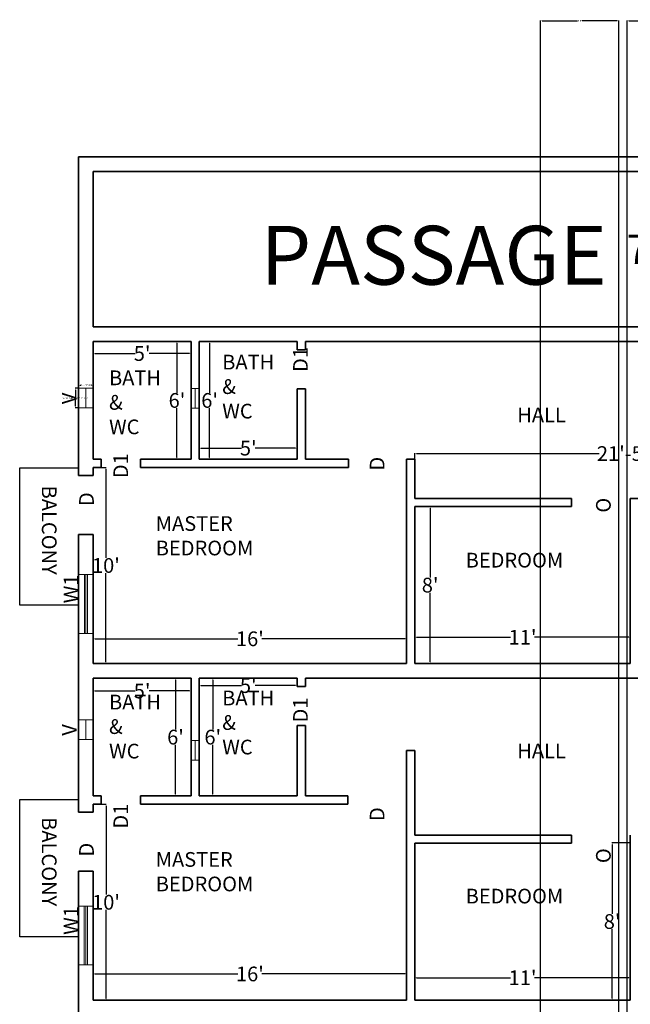
# Model space of a CAD drawing. Units: inches. Extents: x -2189 to 546, y 945 to 2684.
# Tile 4 of 10: x -866 to -492, y 2082 to 2684. Entities that reach past the tile are written whole.
import ezdxf

# ---------------------------------------------------------------- set-up
doc = ezdxf.new("R2010")
doc.units = ezdxf.units.IN
doc.header["$MEASUREMENT"] = 0
for name, color, linetype, lineweight in [('A-ANNO-DIMS', 2, 'Continuous', 13), ('A-ANNO-TEXT', 7, 'Continuous', 18), ('A-AREA-IDEN', 3, 'Continuous', 18), ('A-FLOR-BALC', 8, 'Continuous', 25), ('A-GLAZ', 4, 'Continuous', 18), ('A-WALL', 7, 'Continuous', 35)]:
    doc.layers.add(name, color=color, linetype=linetype, lineweight=lineweight)
doc.styles.get("Standard").update_dxf_attribs({"font": 'arial.ttf'})
doc.dimstyles.get("Standard").update_dxf_attribs({"dimtxt": 1, "dimasz": 1, "dimexe": 0.18, "dimexo": 0.0625, "dimgap": 0.09, "dimtad": 0, "dimtih": 1, "dimtoh": 1, "dimdec": 0, "dimzin": 0, "dimdsep": 46, "dimlunit": 3, "dimtxsty": 'Standard', "dimcen": 0.09, "dimadec": 0, "dimazin": 0, "dimtfac": 1, "dimtdec": 0, "dimtofl": 0, "dimtmove": 0, "dimatfit": 3, "dimfxl": 1, "dimtolj": 1, "dimtzin": 0, "dimarcsym": 0})

# ---------------------------------------------------------------- blocks, each defined once
blk = doc.blocks.new('*D57')
at = {"layer": 'A-ANNO-DIMS', "color": 0, "lineweight": -2, "transparency": 16777216}
for p, q in [((-820.78, 2084.24), (-820.78, 2100.43)), ((-819.78, 2100.25), (-732.08, 2100.25)), ((-629.78, 2100.25), (-717.48, 2100.25)), ((-628.78, 2084.24), (-628.78, 2100.43))]:
    blk.add_line(p, q, dxfattribs=at)
at = {"layer": 'A-ANNO-DIMS', "color": 0, "transparency": 16777216}
for points in [[(-819.78, 2100.42), (-819.78, 2100.08), (-820.78, 2100.25)], [(-629.78, 2100.42), (-629.78, 2100.08), (-628.78, 2100.25)]]:
    blk.add_solid(points, dxfattribs=at)
at = {"layer": 'Defpoints', "color": 0, "transparency": 16777216}
for p in [(-820.78, 2100.25), (-820.78, 2084.17), (-628.78, 2084.17)]:
    blk.add_point(p, dxfattribs=at)
at = {"layer": 'A-ANNO-DIMS', "color": 0, "transparency": 16777216, "insert": (-724.78, 2100.25), "char_height": 1, "attachment_point": 5}
blk.add_mtext("\\A1;{\\H9x;16'}", dxfattribs=at)
blk = doc.blocks.new('*D58')
at = {"layer": 'A-ANNO-DIMS', "color": 0, "lineweight": -2, "transparency": 16777216}
for p, q in [((-623.78, 2084.24), (-623.78, 2098.13)), ((-622.78, 2097.95), (-565.08, 2097.95)), ((-492.78, 2097.95), (-550.48, 2097.95)), ((-491.78, 2084.24), (-491.78, 2098.13))]:
    blk.add_line(p, q, dxfattribs=at)
at = {"layer": 'A-ANNO-DIMS', "color": 0, "transparency": 16777216}
for points in [[(-622.78, 2098.12), (-622.78, 2097.78), (-623.78, 2097.95)], [(-492.78, 2098.12), (-492.78, 2097.78), (-491.78, 2097.95)]]:
    blk.add_solid(points, dxfattribs=at)
at = {"layer": 'Defpoints', "color": 0, "transparency": 16777216}
for p in [(-623.78, 2097.95), (-623.78, 2084.17), (-491.78, 2084.17)]:
    blk.add_point(p, dxfattribs=at)
at = {"layer": 'A-ANNO-DIMS', "color": 0, "transparency": 16777216, "insert": (-557.78, 2097.95), "char_height": 1, "attachment_point": 5}
blk.add_mtext("\\A1;{\\H9x;11'}", dxfattribs=at)
blk = doc.blocks.new('*D61')
at = {"layer": 'A-ANNO-DIMS', "color": 0, "lineweight": -2, "transparency": 16777216}
for p, q in [((-820.78, 2281.11), (-820.78, 2273.2)), ((-760.78, 2281.11), (-760.78, 2273.2)), ((-819.78, 2273.38), (-795.01, 2273.38)), ((-761.78, 2273.38), (-786.55, 2273.38))]:
    blk.add_line(p, q, dxfattribs=at)
at = {"layer": 'A-ANNO-DIMS', "color": 0, "transparency": 16777216}
for points in [[(-819.78, 2273.55), (-819.78, 2273.22), (-820.78, 2273.38)], [(-761.78, 2273.55), (-761.78, 2273.22), (-760.78, 2273.38)]]:
    blk.add_solid(points, dxfattribs=at)
at = {"layer": 'Defpoints', "color": 0, "transparency": 16777216}
for p in [(-820.78, 2281.17), (-760.78, 2281.17), (-820.78, 2273.38)]:
    blk.add_point(p, dxfattribs=at)
at = {"layer": 'A-ANNO-DIMS', "color": 0, "transparency": 16777216, "insert": (-790.78, 2273.38), "char_height": 1, "attachment_point": 5}
blk.add_mtext("\\A1;{\\H9x;5'}", dxfattribs=at)
blk = doc.blocks.new('*D62')
at = {"layer": 'A-ANNO-DIMS', "color": 0, "lineweight": -2, "transparency": 16777216}
for p, q in [((-760.84, 2281.17), (-770.51, 2281.17)), ((-770.33, 2280.17), (-770.33, 2249.86)), ((-770.33, 2210.17), (-770.33, 2240.49)), ((-760.84, 2209.17), (-770.51, 2209.17))]:
    blk.add_line(p, q, dxfattribs=at)
at = {"layer": 'A-ANNO-DIMS', "color": 0, "transparency": 16777216}
for points in [[(-770.5, 2280.17), (-770.17, 2280.17), (-770.33, 2281.17)], [(-770.5, 2210.17), (-770.17, 2210.17), (-770.33, 2209.17)]]:
    blk.add_solid(points, dxfattribs=at)
at = {"layer": 'Defpoints', "color": 0, "transparency": 16777216}
for p in [(-770.33, 2281.17), (-760.78, 2281.17), (-760.78, 2209.17)]:
    blk.add_point(p, dxfattribs=at)
at = {"layer": 'A-ANNO-DIMS', "color": 0, "transparency": 16777216, "insert": (-770.33, 2245.17), "char_height": 1, "attachment_point": 5}
blk.add_mtext("\\A1;{\\H9x;6'}", dxfattribs=at)
blk = doc.blocks.new('*D63')
at = {"layer": 'A-ANNO-DIMS', "color": 0, "lineweight": -2, "transparency": 16777216}
for p, q in [((-755.72, 2281.17), (-747.34, 2281.17)), ((-747.52, 2280.17), (-747.52, 2249.86)), ((-747.52, 2210.17), (-747.52, 2240.49)), ((-755.72, 2209.17), (-747.34, 2209.17))]:
    blk.add_line(p, q, dxfattribs=at)
at = {"layer": 'A-ANNO-DIMS', "color": 0, "transparency": 16777216}
for points in [[(-747.69, 2280.17), (-747.35, 2280.17), (-747.52, 2281.17)], [(-747.69, 2210.17), (-747.35, 2210.17), (-747.52, 2209.17)]]:
    blk.add_solid(points, dxfattribs=at)
at = {"layer": 'Defpoints', "color": 0, "transparency": 16777216}
for p in [(-755.78, 2281.17), (-747.52, 2281.17), (-755.78, 2209.17)]:
    blk.add_point(p, dxfattribs=at)
at = {"layer": 'A-ANNO-DIMS', "color": 0, "transparency": 16777216, "insert": (-747.52, 2245.17), "char_height": 1, "attachment_point": 5}
blk.add_mtext("\\A1;{\\H9x;6'}", dxfattribs=at)
blk = doc.blocks.new('*D64')
at = {"layer": 'A-ANNO-DIMS', "color": 0, "lineweight": -2, "transparency": 16777216}
for p, q in [((-755.78, 2281.11), (-755.78, 2276.52)), ((-695.78, 2281.11), (-695.78, 2276.52)), ((-754.78, 2276.7), (-730.01, 2276.7)), ((-696.78, 2276.7), (-721.55, 2276.7))]:
    blk.add_line(p, q, dxfattribs=at)
at = {"layer": 'A-ANNO-DIMS', "color": 0, "transparency": 16777216}
for points in [[(-754.78, 2276.86), (-754.78, 2276.53), (-755.78, 2276.7)], [(-696.78, 2276.86), (-696.78, 2276.53), (-695.78, 2276.7)]]:
    blk.add_solid(points, dxfattribs=at)
at = {"layer": 'Defpoints', "color": 0, "transparency": 16777216}
for p in [(-755.78, 2281.17), (-695.78, 2281.17), (-755.78, 2276.7)]:
    blk.add_point(p, dxfattribs=at)
at = {"layer": 'A-ANNO-DIMS', "color": 0, "transparency": 16777216, "insert": (-725.78, 2276.7), "char_height": 1, "attachment_point": 5}
blk.add_mtext("\\A1;{\\H9x;5'}", dxfattribs=at)
blk = doc.blocks.new('*D65')
at = {"layer": 'A-ANNO-DIMS', "color": 0, "lineweight": -2, "transparency": 16777216}
for p, q in [((-820.75, 2204.04), (-812.72, 2204.04)), ((-812.9, 2203.04), (-812.9, 2148.8)), ((-812.9, 2085.19), (-812.9, 2139.43)), ((-820.75, 2084.19), (-812.72, 2084.19))]:
    blk.add_line(p, q, dxfattribs=at)
at = {"layer": 'A-ANNO-DIMS', "color": 0, "transparency": 16777216}
for points in [[(-813.07, 2203.04), (-812.73, 2203.04), (-812.9, 2204.04)], [(-813.07, 2085.19), (-812.73, 2085.19), (-812.9, 2084.19)]]:
    blk.add_solid(points, dxfattribs=at)
at = {"layer": 'Defpoints', "color": 0, "transparency": 16777216}
for p in [(-820.82, 2204.04), (-820.82, 2084.19), (-812.9, 2084.19)]:
    blk.add_point(p, dxfattribs=at)
at = {"layer": 'A-ANNO-DIMS', "color": 0, "transparency": 16777216, "insert": (-812.9, 2144.11), "char_height": 1, "attachment_point": 5}
blk.add_mtext("\\A1;{\\H9x;10'}", dxfattribs=at)
blk = doc.blocks.new('*D66')
at = {"layer": 'A-ANNO-DIMS', "color": 0, "lineweight": -2, "transparency": 16777216}
for p, q in [((-491.84, 2180.47), (-503.11, 2180.47)), ((-502.93, 2179.47), (-502.93, 2137.01)), ((-502.93, 2085.17), (-502.93, 2127.64)), ((-491.84, 2084.17), (-503.11, 2084.17))]:
    blk.add_line(p, q, dxfattribs=at)
at = {"layer": 'A-ANNO-DIMS', "color": 0, "transparency": 16777216}
for points in [[(-503.1, 2179.47), (-502.76, 2179.47), (-502.93, 2180.47)], [(-503.1, 2085.17), (-502.76, 2085.17), (-502.93, 2084.17)]]:
    blk.add_solid(points, dxfattribs=at)
at = {"layer": 'Defpoints', "color": 0, "transparency": 16777216}
for p in [(-491.78, 2180.47), (-502.93, 2084.17), (-491.78, 2084.17)]:
    blk.add_point(p, dxfattribs=at)
at = {"layer": 'A-ANNO-DIMS', "color": 0, "transparency": 16777216, "insert": (-502.93, 2132.32), "char_height": 1, "attachment_point": 5}
blk.add_mtext("\\A1;{\\H9x;8'}", dxfattribs=at)
blk = doc.blocks.new('*D67')
at = {"layer": 'A-ANNO-DIMS', "color": 0, "lineweight": -2, "transparency": 16777216}
for p, q in [((-820.78, 2290.24), (-820.78, 2305.51)), ((-819.78, 2305.33), (-732.08, 2305.33)), ((-629.78, 2305.33), (-717.48, 2305.33)), ((-628.78, 2290.24), (-628.78, 2305.51))]:
    blk.add_line(p, q, dxfattribs=at)
at = {"layer": 'A-ANNO-DIMS', "color": 0, "transparency": 16777216}
for points in [[(-819.78, 2305.5), (-819.78, 2305.17), (-820.78, 2305.33)], [(-629.78, 2305.5), (-629.78, 2305.17), (-628.78, 2305.33)]]:
    blk.add_solid(points, dxfattribs=at)
at = {"layer": 'Defpoints', "color": 0, "transparency": 16777216}
for p in [(-820.78, 2305.33), (-820.78, 2290.17), (-628.78, 2290.17)]:
    blk.add_point(p, dxfattribs=at)
at = {"layer": 'A-ANNO-DIMS', "color": 0, "transparency": 16777216, "insert": (-724.78, 2305.33), "char_height": 1, "attachment_point": 5}
blk.add_mtext("\\A1;{\\H9x;16'}", dxfattribs=at)
blk = doc.blocks.new('*D68')
at = {"layer": 'A-ANNO-DIMS', "color": 0, "lineweight": -2, "transparency": 16777216}
for p, q in [((-623.78, 2290.24), (-623.78, 2306.45)), ((-622.78, 2306.27), (-565.08, 2306.27)), ((-492.78, 2306.27), (-550.48, 2306.27)), ((-491.78, 2290.24), (-491.78, 2306.45))]:
    blk.add_line(p, q, dxfattribs=at)
at = {"layer": 'A-ANNO-DIMS', "color": 0, "transparency": 16777216}
for points in [[(-622.78, 2306.44), (-622.78, 2306.1), (-623.78, 2306.27)], [(-492.78, 2306.44), (-492.78, 2306.1), (-491.78, 2306.27)]]:
    blk.add_solid(points, dxfattribs=at)
at = {"layer": 'Defpoints', "color": 0, "transparency": 16777216}
for p in [(-623.78, 2306.27), (-623.78, 2290.17), (-491.78, 2290.17)]:
    blk.add_point(p, dxfattribs=at)
at = {"layer": 'A-ANNO-DIMS', "color": 0, "transparency": 16777216, "insert": (-557.78, 2306.27), "char_height": 1, "attachment_point": 5}
blk.add_mtext("\\A1;{\\H9x;11'}", dxfattribs=at)
blk = doc.blocks.new('*D69')
at = {"layer": 'A-ANNO-DIMS', "color": 0, "lineweight": -2, "transparency": 16777216}
for p, q in [((-623.72, 2386.17), (-614.2, 2386.17)), ((-614.38, 2385.17), (-614.38, 2342.86)), ((-614.38, 2291.17), (-614.38, 2333.49)), ((-623.72, 2290.17), (-614.2, 2290.17))]:
    blk.add_line(p, q, dxfattribs=at)
at = {"layer": 'A-ANNO-DIMS', "color": 0, "transparency": 16777216}
for points in [[(-614.55, 2385.17), (-614.21, 2385.17), (-614.38, 2386.17)], [(-614.55, 2291.17), (-614.21, 2291.17), (-614.38, 2290.17)]]:
    blk.add_solid(points, dxfattribs=at)
at = {"layer": 'Defpoints', "color": 0, "transparency": 16777216}
for p in [(-623.78, 2386.17), (-614.38, 2386.17), (-623.78, 2290.17)]:
    blk.add_point(p, dxfattribs=at)
at = {"layer": 'A-ANNO-DIMS', "color": 0, "transparency": 16777216, "insert": (-614.38, 2338.17), "char_height": 1, "attachment_point": 5}
blk.add_mtext("\\A1;{\\H9x;8'}", dxfattribs=at)
blk = doc.blocks.new('*D72')
at = {"layer": 'A-ANNO-DIMS', "color": 0, "lineweight": -2, "transparency": 16777216}
for p, q in [((-820.72, 2410.17), (-812.77, 2410.17)), ((-812.95, 2409.17), (-812.95, 2354.86)), ((-812.95, 2291.17), (-812.95, 2345.49)), ((-820.72, 2290.17), (-812.77, 2290.17))]:
    blk.add_line(p, q, dxfattribs=at)
at = {"layer": 'A-ANNO-DIMS', "color": 0, "transparency": 16777216}
for points in [[(-813.12, 2409.17), (-812.78, 2409.17), (-812.95, 2410.17)], [(-813.12, 2291.17), (-812.78, 2291.17), (-812.95, 2290.17)]]:
    blk.add_solid(points, dxfattribs=at)
at = {"layer": 'Defpoints', "color": 0, "transparency": 16777216}
for p in [(-820.78, 2410.17), (-812.95, 2410.17), (-820.78, 2290.17)]:
    blk.add_point(p, dxfattribs=at)
at = {"layer": 'A-ANNO-DIMS', "color": 0, "transparency": 16777216, "insert": (-812.95, 2350.17), "char_height": 1, "attachment_point": 5}
blk.add_mtext("\\A1;{\\H9x;10'}", dxfattribs=at)
blk = doc.blocks.new('*D73')
at = {"layer": 'A-ANNO-DIMS', "color": 0, "lineweight": -2, "transparency": 16777216}
for p, q in [((-820.78, 2487.11), (-820.78, 2479.7)), ((-760.78, 2487.11), (-760.78, 2479.7)), ((-819.78, 2479.88), (-795.01, 2479.88)), ((-761.78, 2479.88), (-786.55, 2479.88))]:
    blk.add_line(p, q, dxfattribs=at)
at = {"layer": 'A-ANNO-DIMS', "color": 0, "transparency": 16777216}
for points in [[(-819.78, 2480.05), (-819.78, 2479.72), (-820.78, 2479.88)], [(-761.78, 2480.05), (-761.78, 2479.72), (-760.78, 2479.88)]]:
    blk.add_solid(points, dxfattribs=at)
at = {"layer": 'Defpoints', "color": 0, "transparency": 16777216}
for p in [(-820.78, 2487.17), (-760.78, 2487.17), (-760.78, 2479.88)]:
    blk.add_point(p, dxfattribs=at)
at = {"layer": 'A-ANNO-DIMS', "color": 0, "transparency": 16777216, "insert": (-790.78, 2479.88), "char_height": 1, "attachment_point": 5}
blk.add_mtext("\\A1;{\\H9x;5'}", dxfattribs=at)
blk = doc.blocks.new('*D74')
at = {"layer": 'A-ANNO-DIMS', "color": 0, "lineweight": -2, "transparency": 16777216}
for p, q in [((-760.84, 2487.17), (-769.63, 2487.17)), ((-769.45, 2486.17), (-769.45, 2455.86)), ((-769.45, 2416.17), (-769.45, 2446.49)), ((-760.84, 2415.17), (-769.63, 2415.17))]:
    blk.add_line(p, q, dxfattribs=at)
at = {"layer": 'A-ANNO-DIMS', "color": 0, "transparency": 16777216}
for points in [[(-769.62, 2486.17), (-769.28, 2486.17), (-769.45, 2487.17)], [(-769.62, 2416.17), (-769.28, 2416.17), (-769.45, 2415.17)]]:
    blk.add_solid(points, dxfattribs=at)
at = {"layer": 'Defpoints', "color": 0, "transparency": 16777216}
for p in [(-769.45, 2487.17), (-760.78, 2487.17), (-760.78, 2415.17)]:
    blk.add_point(p, dxfattribs=at)
at = {"layer": 'A-ANNO-DIMS', "color": 0, "transparency": 16777216, "insert": (-769.45, 2451.17), "char_height": 1, "attachment_point": 5}
blk.add_mtext("\\A1;{\\H9x;6'}", dxfattribs=at)
blk = doc.blocks.new('*D75')
at = {"layer": 'A-ANNO-DIMS', "color": 0, "lineweight": -2, "transparency": 16777216}
for p, q in [((-755.72, 2487.17), (-749.27, 2487.17)), ((-749.45, 2486.17), (-749.45, 2455.86)), ((-749.45, 2416.17), (-749.45, 2446.49)), ((-755.72, 2415.17), (-749.27, 2415.17))]:
    blk.add_line(p, q, dxfattribs=at)
at = {"layer": 'A-ANNO-DIMS', "color": 0, "transparency": 16777216}
for points in [[(-749.61, 2486.17), (-749.28, 2486.17), (-749.45, 2487.17)], [(-749.61, 2416.17), (-749.28, 2416.17), (-749.45, 2415.17)]]:
    blk.add_solid(points, dxfattribs=at)
at = {"layer": 'Defpoints', "color": 0, "transparency": 16777216}
for p in [(-755.78, 2487.17), (-749.45, 2487.17), (-755.78, 2415.17)]:
    blk.add_point(p, dxfattribs=at)
at = {"layer": 'A-ANNO-DIMS', "color": 0, "transparency": 16777216, "insert": (-749.45, 2451.17), "char_height": 1, "attachment_point": 5}
blk.add_mtext("\\A1;{\\H9x;6'}", dxfattribs=at)
blk = doc.blocks.new('*D76')
at = {"layer": 'A-ANNO-DIMS', "color": 0, "lineweight": -2, "transparency": 16777216}
for p, q in [((-755.78, 2415.24), (-755.78, 2422.17)), ((-754.78, 2421.99), (-730.01, 2421.99)), ((-696.78, 2421.99), (-721.55, 2421.99)), ((-695.78, 2415.24), (-695.78, 2422.17))]:
    blk.add_line(p, q, dxfattribs=at)
at = {"layer": 'A-ANNO-DIMS', "color": 0, "transparency": 16777216}
for points in [[(-754.78, 2422.15), (-754.78, 2421.82), (-755.78, 2421.99)], [(-696.78, 2422.15), (-696.78, 2421.82), (-695.78, 2421.99)]]:
    blk.add_solid(points, dxfattribs=at)
at = {"layer": 'Defpoints', "color": 0, "transparency": 16777216}
for p in [(-695.78, 2421.99), (-755.78, 2415.17), (-695.78, 2415.17)]:
    blk.add_point(p, dxfattribs=at)
at = {"layer": 'A-ANNO-DIMS', "color": 0, "transparency": 16777216, "insert": (-725.78, 2421.99), "char_height": 1, "attachment_point": 5}
blk.add_mtext("\\A1;{\\H9x;5'}", dxfattribs=at)
blk = doc.blocks.new('*D77')
at = {"layer": 'A-ANNO-DIMS', "color": 0, "lineweight": -2, "transparency": 16777216}
for p, q in [((-623.78, 2415.24), (-623.78, 2418.85)), ((-622.78, 2418.67), (-510.9, 2418.67)), ((-367.78, 2418.67), (-479.65, 2418.67)), ((-366.78, 2415.24), (-366.78, 2418.85))]:
    blk.add_line(p, q, dxfattribs=at)
at = {"layer": 'A-ANNO-DIMS', "color": 0, "transparency": 16777216}
for points in [[(-622.78, 2418.84), (-622.78, 2418.51), (-623.78, 2418.67)], [(-367.78, 2418.84), (-367.78, 2418.51), (-366.78, 2418.67)]]:
    blk.add_solid(points, dxfattribs=at)
at = {"layer": 'Defpoints', "color": 0, "transparency": 16777216}
for p in [(-366.78, 2418.67), (-623.78, 2415.17), (-366.78, 2415.17)]:
    blk.add_point(p, dxfattribs=at)
at = {"layer": 'A-ANNO-DIMS', "color": 0, "transparency": 16777216, "insert": (-495.28, 2418.67), "char_height": 1, "attachment_point": 5}
blk.add_mtext('\\A1;{\\H9x;21\'-5"}', dxfattribs=at)
blk = doc.blocks.new('*D84')
at = {"layer": 'A-ANNO-DIMS', "color": 0, "lineweight": -2, "transparency": 16777216}
for p, q in [((-452.79, 2591.17), (-460.17, 2591.17)), ((-459.99, 2590.17), (-459.99, 2552.8)), ((-459.99, 2497.17), (-459.99, 2534.55)), ((-452.79, 2496.17), (-460.17, 2496.17))]:
    blk.add_line(p, q, dxfattribs=at)
at = {"layer": 'A-ANNO-DIMS', "color": 0, "transparency": 16777216}
for points in [[(-460.16, 2590.17), (-459.83, 2590.17), (-459.99, 2591.17)], [(-460.16, 2497.17), (-459.83, 2497.17), (-459.99, 2496.17)]]:
    blk.add_solid(points, dxfattribs=at)
at = {"layer": 'Defpoints', "color": 0, "transparency": 16777216}
for p in [(-452.73, 2591.17), (-459.99, 2496.17), (-452.73, 2496.17)]:
    blk.add_point(p, dxfattribs=at)
at = {"layer": 'A-ANNO-DIMS', "color": 0, "transparency": 16777216, "insert": (-459.99, 2543.67), "char_height": 1, "attachment_point": 5}
blk.add_mtext('\\A1;{\\H18x;7\'-11"}', dxfattribs=at)
blk = doc.blocks.new('WIN-36X9')
for p, q in [((0, 5.5), (36, 5.5)), ((0, 5.5), (36, 5.5)), ((0, 4.5), (36, 4.5)), ((0, 3.5), (36, 3.5))]:
    blk.add_line(p, q)
blk.add_lwpolyline([(0, 0), (0, 9), (36, 9), (36, 0)], close=True)
blk = doc.blocks.new('VENT-12X5')
blk.add_line((2.5, 12), (2.5, 0))
blk.add_lwpolyline([(5, 12), (0, 12), (0, 0), (5, 0)], close=True)
blk = doc.blocks.new('VENT-12X9-SINGLELINE')
blk.add_line((4.5, 12), (4.5, 0))
blk.add_lwpolyline([(0, 12), (9, 12), (9, 0), (0, 0)], close=True)
blk = doc.blocks.new('BALCONY-36X84')
for p, q in [((0, 0), (0, 84)), ((0, 84), (36, 84)), ((36, 0), (0, 0))]:
    blk.add_line(p, q)
blk = doc.blocks.new('*D97')
at = {"layer": 'A-ANNO-DIMS', "color": 0, "lineweight": -2, "transparency": 16777216}
for p, q in [((-829.84, 2458.62), (-831.76, 2458.62)), ((-831.58, 2457.62), (-831.58, 2453.36)), ((-829.84, 2446.62), (-831.76, 2446.62)), ((-831.58, 2447.62), (-831.58, 2451.87))]:
    blk.add_line(p, q, dxfattribs=at)
at = {"layer": 'A-ANNO-DIMS', "color": 0, "transparency": 16777216}
for points in [[(-831.75, 2457.62), (-831.41, 2457.62), (-831.58, 2458.62)], [(-831.75, 2447.62), (-831.41, 2447.62), (-831.58, 2446.62)]]:
    blk.add_solid(points, dxfattribs=at)
at = {"layer": 'Defpoints', "color": 0, "transparency": 16777216}
for p in [(-831.58, 2458.62), (-829.78, 2458.62), (-829.78, 2446.62)]:
    blk.add_point(p, dxfattribs=at)
at = {"layer": 'A-ANNO-DIMS', "color": 0, "transparency": 16777216, "insert": (-831.58, 2452.62), "char_height": 1, "attachment_point": 5}
blk.add_mtext('\\A1;VENT (SINGLE) 1\'-0" TYP.', dxfattribs=at)
blk = doc.blocks.new('*D98')
at = {"layer": 'A-ANNO-DIMS', "color": 0, "lineweight": -2, "transparency": 16777216}
for p, q in [((-829.78, 2458.68), (-829.78, 2460.6)), ((-828.78, 2460.42), (-828.42, 2460.42)), ((-821.78, 2460.42), (-822.14, 2460.42)), ((-820.78, 2458.68), (-820.78, 2460.6))]:
    blk.add_line(p, q, dxfattribs=at)
at = {"layer": 'A-ANNO-DIMS', "color": 0, "transparency": 16777216}
for points in [[(-828.78, 2460.58), (-828.78, 2460.25), (-829.78, 2460.42)], [(-821.78, 2460.58), (-821.78, 2460.25), (-820.78, 2460.42)]]:
    blk.add_solid(points, dxfattribs=at)
at = {"layer": 'Defpoints', "color": 0, "transparency": 16777216}
for p in [(-829.78, 2458.62), (-820.78, 2460.42), (-820.78, 2458.62)]:
    blk.add_point(p, dxfattribs=at)
at = {"layer": 'A-ANNO-DIMS', "color": 0, "transparency": 16777216, "insert": (-825.28, 2460.42), "char_height": 1, "attachment_point": 5}
blk.add_mtext('\\A1;0\'-9" TYP.', dxfattribs=at)
blk = doc.blocks.new('*D104')
at = {"layer": 'A-ANNO-DIMS', "color": 0, "lineweight": -2, "transparency": 16777216}
for p, q in [((-493.78, 1873.24), (-493.78, 2683.65)), ((-492.78, 2683.47), (-449.69, 2683.47)), ((-403.78, 2683.47), (-446.86, 2683.47)), ((-402.78, 1873.24), (-402.78, 2683.65))]:
    blk.add_line(p, q, dxfattribs=at)
at = {"layer": 'A-ANNO-DIMS', "color": 0, "transparency": 16777216}
for points in [[(-492.78, 2683.64), (-492.78, 2683.31), (-493.78, 2683.47)], [(-403.78, 2683.64), (-403.78, 2683.31), (-402.78, 2683.47)]]:
    blk.add_solid(points, dxfattribs=at)
at = {"layer": 'Defpoints', "color": 0, "transparency": 16777216}
for p in [(-402.78, 2683.47), (-493.78, 1873.17), (-402.78, 1873.17)]:
    blk.add_point(p, dxfattribs=at)
at = {"layer": 'A-ANNO-DIMS', "color": 0, "transparency": 16777216, "insert": (-448.28, 2683.47), "char_height": 1, "attachment_point": 5}
blk.add_mtext('\\A1;7\'-7"', dxfattribs=at)
blk = doc.blocks.new('*D106')
at = {"layer": 'A-ANNO-DIMS', "color": 0, "lineweight": -2, "transparency": 16777216}
for p, q in [((-546.78, 1832.24), (-546.78, 2683.65)), ((-545.78, 2683.47), (-524.22, 2683.47)), ((-499.78, 2683.47), (-521.34, 2683.47)), ((-498.78, 1832.24), (-498.78, 2683.65))]:
    blk.add_line(p, q, dxfattribs=at)
at = {"layer": 'A-ANNO-DIMS', "color": 0, "transparency": 16777216}
for points in [[(-545.78, 2683.64), (-545.78, 2683.31), (-546.78, 2683.47)], [(-499.78, 2683.64), (-499.78, 2683.31), (-498.78, 2683.47)]]:
    blk.add_solid(points, dxfattribs=at)
at = {"layer": 'Defpoints', "color": 0, "transparency": 16777216}
for p in [(-498.78, 2683.47), (-546.78, 1832.17), (-498.78, 1832.17)]:
    blk.add_point(p, dxfattribs=at)
at = {"layer": 'A-ANNO-DIMS', "color": 0, "transparency": 16777216, "insert": (-522.78, 2683.47), "char_height": 1, "attachment_point": 5}
blk.add_mtext('\\A1;4\'-0"', dxfattribs=at)

msp = doc.modelspace()

# ---------------------------------------------------------------- linework, layer by layer
at = {"layer": 'A-GLAZ'}
for p, q in [((-826.11, 2308.61), (-826.11, 2344.61)), ((-825.28, 2308.61), (-825.28, 2344.61)), ((-824.28, 2308.61), (-824.28, 2344.61))]:
    msp.add_line(p, q, dxfattribs=at)
msp.add_lwpolyline([(-820.78, 2308.61), (-829.78, 2308.61), (-829.78, 2344.61), (-820.78, 2344.61)], close=True, dxfattribs=at)
at = {"layer": 'A-WALL'}
for p, q in [((-829.78, 2600.17), (-262.78, 2600.17)), ((-829.78, 2405.17), (-829.78, 2600.17)), ((-820.78, 2591.17), (-271.78, 2591.17)), ((-820.78, 2496.17), (-820.78, 2591.17)), ((-755.78, 2496.17), (-820.78, 2496.17)), ((-357.78, 2496.17), (-755.78, 2496.17)), ((-820.78, 2415.17), (-820.78, 2487.17)), ((-760.78, 2487.17), (-820.78, 2487.17)), ((-760.78, 2415.17), (-760.78, 2487.17)), ((-755.78, 2415.17), (-755.78, 2487.17)), ((-695.78, 2487.17), (-755.78, 2487.17)), ((-695.78, 2482.17), (-695.78, 2487.17)), ((-695.78, 2482.17), (-690.78, 2482.17)), ((-366.78, 2487.17), (-690.78, 2487.17)), ((-690.78, 2482.17), (-690.78, 2487.17)), ((-695.78, 2415.17), (-695.78, 2458.17)), ((-695.78, 2458.17), (-690.78, 2458.17)), ((-690.78, 2415.17), (-690.78, 2458.17)), ((-815.78, 2415.17), (-820.78, 2415.17)), ((-820.78, 2405.17), (-820.78, 2410.17)), ((-815.78, 2410.17), (-820.78, 2410.17)), ((-815.78, 2415.17), (-815.78, 2410.17)), ((-760.78, 2415.17), (-791.78, 2415.17)), ((-791.78, 2415.17), (-791.78, 2410.17)), ((-664.46, 2410.17), (-791.78, 2410.17)), ((-695.78, 2415.17), (-755.78, 2415.17)), ((-664.46, 2415.17), (-690.78, 2415.17)), ((-664.46, 2410.17), (-664.46, 2415.17)), ((-623.78, 2415.17), (-628.78, 2415.17)), ((-628.78, 2410.17), (-628.78, 2415.17)), ((-628.78, 2290.17), (-628.78, 2410.17)), ((-623.78, 2391.17), (-623.78, 2415.17)), ((-820.78, 2405.17), (-829.78, 2405.17)), ((-527.78, 2391.17), (-623.78, 2391.17)), ((-623.78, 2290.17), (-623.78, 2386.17)), ((-527.78, 2386.17), (-623.78, 2386.17)), ((-527.78, 2386.17), (-527.78, 2391.17)), ((-491.78, 2386.17), (-491.78, 2391.17)), ((-481.78, 2391.17), (-491.78, 2391.17)), ((-491.78, 2290.17), (-491.78, 2386.17)), ((-829.78, 2199.17), (-829.78, 2369.17)), ((-820.78, 2369.17), (-829.78, 2369.17)), ((-820.78, 2290.17), (-820.78, 2369.17)), ((-628.78, 2290.17), (-820.78, 2290.17)), ((-491.78, 2290.17), (-623.78, 2290.17)), ((-820.78, 2209.17), (-820.78, 2281.17)), ((-760.78, 2281.17), (-820.78, 2281.17)), ((-760.78, 2209.17), (-760.78, 2281.17)), ((-755.78, 2209.17), (-755.78, 2281.17)), ((-695.78, 2281.17), (-755.78, 2281.17)), ((-695.78, 2276.17), (-695.78, 2281.17)), ((-366.78, 2281.17), (-690.78, 2281.17)), ((-690.78, 2276.17), (-690.78, 2281.17)), ((-695.78, 2276.17), (-690.78, 2276.17)), ((-695.78, 2209.17), (-695.78, 2252.17)), ((-695.78, 2252.17), (-690.78, 2252.17)), ((-690.78, 2209.17), (-690.78, 2252.17)), ((-628.78, 2209.17), (-628.78, 2236.96)), ((-628.78, 2236.96), (-623.78, 2236.96)), ((-623.78, 2185.17), (-623.78, 2236.96)), ((-815.78, 2209.17), (-820.78, 2209.17)), ((-815.78, 2209.17), (-815.78, 2204.17)), ((-760.78, 2209.17), (-791.78, 2209.17)), ((-791.78, 2209.17), (-791.78, 2204.17)), ((-695.78, 2209.17), (-755.78, 2209.17)), ((-664.78, 2209.17), (-690.78, 2209.17)), ((-664.78, 2204.17), (-664.78, 2209.17)), ((-628.78, 2204.17), (-628.78, 2209.17)), ((-820.78, 2199.17), (-829.78, 2199.17)), ((-820.78, 2199.17), (-820.78, 2204.17)), ((-815.78, 2204.17), (-820.78, 2204.17)), ((-664.78, 2204.17), (-791.78, 2204.17)), ((-628.78, 2084.17), (-628.78, 2204.17)), ((-527.78, 2185.17), (-623.78, 2185.17)), ((-527.78, 2180.17), (-527.78, 2185.17)), ((-491.78, 2084.17), (-491.78, 2185.17)), ((-623.78, 2084.17), (-623.78, 2180.17)), ((-527.78, 2180.17), (-623.78, 2180.17)), ((-829.78, 1997.17), (-829.78, 2163.17)), ((-820.78, 2163.17), (-829.78, 2163.17)), ((-820.78, 2084.17), (-820.78, 2163.17)), ((-628.78, 2084.17), (-820.78, 2084.17)), ((-491.78, 2084.17), (-623.78, 2084.17))]:
    msp.add_line(p, q, dxfattribs=at)

# ---------------------------------------------------------------- block references
at = {"layer": 'A-FLOR-BALC'}
for p in [(-865.78, 2325.87), (-865.78, 2123.01)]:
    msp.add_blockref('BALCONY-36X84', p, dxfattribs=at)
at = {"layer": 'A-GLAZ'}
for name, p in [('VENT-12X9-SINGLELINE', (-829.78, 2446.62)), ('VENT-12X5', (-760.78, 2446.38)), ('VENT-12X9-SINGLELINE', (-829.78, 2243.76)), ('VENT-12X5', (-760.78, 2231.03))]:
    msp.add_blockref(name, p, dxfattribs=at)
at = {"layer": 'A-GLAZ', "rotation": 90.00000000000175}
msp.add_blockref('WIN-36X9', (-820.78, 2105.75), dxfattribs=at)

# ---------------------------------------------------------------- texts
at = {"layer": 'A-ANNO-TEXT', "char_height": 9, "attachment_point": 1, "rotation": 90}
for s, width, heights, insert in [('D1', 15.3658, [0], (-698.32, 2468.57)), ('V', 17.5973, [0], (-839.88, 2448.87)), ('D1', 15.3658, [0], (-808.38, 2403.59)), ('D', 15.3658, [0], (-651.37, 2408.24)), ('D', 15.3658, [0], (-829.35, 2386.52)), ('O', 18.6541, [0.207], (-512.78, 2382.5)), ('W1', 11.3125, [0], (-838.78, 2327.04)), ('D1', 15.3658, [0], (-698.32, 2254.13)), ('V', 17.5973, [0], (-839.88, 2246.01)), ('D1', 15.3658, [0], (-808.38, 2189.15)), ('D', 15.3658, [0], (-651.37, 2193.8)), ('D', 15.3658, [0], (-829.35, 2172.08)), ('O', 18.6541, [0.207], (-512.78, 2168.05)), ('W1', 11.3125, [0], (-838.78, 2124.18))]:
    msp.add_mtext_dynamic_manual_height_columns(s, width=width, gutter_width=1, heights=heights, dxfattribs=dict(at, insert=insert))
at = {"layer": 'A-AREA-IDEN', "attachment_point": 1}
for s, width, heights, insert, char_height in [('PASSAGE', 260.6717, [220.33], (-718.3, 2557.99), 36), ('BATH \\P& \\PWC', 29.3144, [0], (-741.71, 2479.13), 9), ('BATH \\P& \\PWC', 29.3144, [0], (-811.04, 2469.49), 9), ('HALL', 37.3459, [0], (-561.01, 2446.77), 9), ('MASTER BEDROOM', 73.5764, [0], (-782.43, 2380.35), 9), ('BEDROOM', 73.8205, [0.207], (-592.63, 2357.93), 9), ('BATH \\P& \\PWC', 29.3144, [0], (-741.71, 2273.59), 9), ('BATH \\P& \\PWC', 29.3144, [0], (-811.04, 2271.1), 9), ('HALL', 37.3459, [0], (-561.01, 2241.23), 9), ('MASTER BEDROOM', 73.5764, [0], (-782.43, 2174.81), 9), ('BEDROOM', 73.8205, [0.207], (-592.63, 2152.39), 9)]:
    msp.add_mtext_dynamic_manual_height_columns(s, width=width, gutter_width=1, heights=heights, dxfattribs=dict(at, insert=insert, char_height=char_height))
at = {"layer": 'A-AREA-IDEN', "char_height": 9, "attachment_point": 1, "rotation": 270}
for insert in [(-843.17, 2399.05), (-843.17, 2196.19)]:
    msp.add_mtext_dynamic_manual_height_columns('BALCONY', width=7.0599, gutter_width=1, heights=[0], dxfattribs=dict(at, insert=insert))

# ---------------------------------------------------------------- dimensions: what is measured, and where the dimension line sits
at = {"layer": 'A-ANNO-DIMS'}
for base, p1, p2, picture, middle in [((-498.78, 2683.47), (-546.78, 1832.17), (-498.78, 1832.17), '*D106', (-522.78, 2683.47)), ((-402.78, 2683.47), (-493.78, 1873.17), (-402.78, 1873.17), '*D104', (-448.28, 2683.47))]:
    dim = msp.add_linear_dim(base=base, p1=p1, p2=p2, dimstyle='Standard', override={"dimdec": 1, "dimlfac": 1, "dimrnd": 0, "dimzin": 1, "dimdsep": 46, "dimlunit": 4, "dimfrac": 2}, dxfattribs=at)
    dim.commit()
    dim.dimension.update_dxf_attribs({"geometry": picture, "text_midpoint": middle})
for base, p1, p2, angle, text, override, picture, middle in [((-459.99, 2496.17), (-452.73, 2591.17), (-452.73, 2496.17), 90, '{\\H18x;<>}', {"dimclrd": 0, "dimclre": 0, "dimclrt": 0}, '*D84', (-459.99, 2543.67)), ((-760.78, 2479.88), (-820.78, 2487.17), (-760.78, 2487.17), 180, '{\\H9x;<>}', {"dimclrd": 0, "dimclre": 0, "dimclrt": 0}, '*D73', (-790.78, 2479.88)), ((-769.45, 2487.17), (-760.78, 2415.17), (-760.78, 2487.17), 90, '{\\H9x;<>}', {"dimclrd": 0, "dimclre": 0, "dimclrt": 0}, '*D74', (-769.45, 2451.17)), ((-749.45, 2487.17), (-755.78, 2415.17), (-755.78, 2487.17), 90, '{\\H9x;<>}', {"dimclrd": 0, "dimclre": 0, "dimclrt": 0}, '*D75', (-749.45, 2451.17)), ((-831.58, 2458.62), (-829.78, 2446.62), (-829.78, 2458.62), 90, 'VENT (SINGLE) <> TYP.', {"dimdec": 1, "dimlfac": 1, "dimrnd": 0, "dimzin": 1, "dimdsep": 46, "dimlunit": 4, "dimfrac": 2}, '*D97', (-831.58, 2452.62)), ((-695.78, 2421.99), (-755.78, 2415.17), (-695.78, 2415.17), 180, '{\\H9x;<>}', {"dimclrd": 0, "dimclre": 0, "dimclrt": 0}, '*D76', (-725.78, 2421.99)), ((-366.78, 2418.67), (-623.78, 2415.17), (-366.78, 2415.17), 180, '{\\H9x;<>}', {"dimclrd": 0, "dimclre": 0, "dimclrt": 0}, '*D77', (-495.28, 2418.67)), ((-614.38, 2386.17), (-623.78, 2290.17), (-623.78, 2386.17), 90, '{\\H9x;<>}', {"dimclrd": 0, "dimclre": 0, "dimclrt": 0}, '*D69', (-614.38, 2338.17)), ((-820.78, 2305.33), (-628.78, 2290.17), (-820.78, 2290.17), 180, '{\\H9x;<>}', {"dimclrd": 0, "dimclre": 0, "dimclrt": 0}, '*D67', (-724.78, 2305.33)), ((-623.78, 2306.27), (-491.78, 2290.17), (-623.78, 2290.17), 180, '{\\H9x;<>}', {"dimclrd": 0, "dimclre": 0, "dimclrt": 0}, '*D68', (-557.78, 2306.27)), ((-820.78, 2273.38), (-760.78, 2281.17), (-820.78, 2281.17), 180, '{\\H9x;<>}', {"dimclrd": 0, "dimclre": 0, "dimclrt": 0}, '*D61', (-790.78, 2273.38)), ((-770.33, 2281.17), (-760.78, 2209.17), (-760.78, 2281.17), 90, '{\\H9x;<>}', {"dimclrd": 0, "dimclre": 0, "dimclrt": 0}, '*D62', (-770.33, 2245.17)), ((-755.78, 2276.7), (-695.78, 2281.17), (-755.78, 2281.17), 180, '{\\H9x;<>}', {"dimclrd": 0, "dimclre": 0, "dimclrt": 0}, '*D64', (-725.78, 2276.7)), ((-747.52, 2281.17), (-755.78, 2209.17), (-755.78, 2281.17), 90, '{\\H9x;<>}', {"dimclrd": 0, "dimclre": 0, "dimclrt": 0}, '*D63', (-747.52, 2245.17)), ((-812.9, 2084.19), (-820.82, 2204.04), (-820.82, 2084.19), 90, '{\\H9x;<>}', {"dimclrd": 0, "dimclre": 0, "dimclrt": 0}, '*D65', (-812.9, 2144.11)), ((-502.93, 2084.17), (-491.78, 2180.47), (-491.78, 2084.17), 90, '{\\H9x;<>}', {"dimclrd": 0, "dimclre": 0, "dimclrt": 0}, '*D66', (-502.93, 2132.32)), ((-820.78, 2100.25), (-628.78, 2084.17), (-820.78, 2084.17), 180, '{\\H9x;<>}', {"dimclrd": 0, "dimclre": 0, "dimclrt": 0}, '*D57', (-724.78, 2100.25)), ((-623.78, 2097.95), (-491.78, 2084.17), (-623.78, 2084.17), 180, '{\\H9x;<>}', {"dimclrd": 0, "dimclre": 0, "dimclrt": 0}, '*D58', (-557.78, 2097.95))]:
    dim = msp.add_linear_dim(base=base, p1=p1, p2=p2, angle=angle, text=text, dimstyle='Standard', override=override, dxfattribs=at)
    dim.commit()
    dim.dimension.update_dxf_attribs({"geometry": picture, "text_midpoint": middle})
dim = msp.add_linear_dim(base=(-820.78, 2460.42), p1=(-829.78, 2458.62), p2=(-820.78, 2458.62), text='<> TYP.', dimstyle='Standard', override={"dimdec": 1, "dimlfac": 1, "dimrnd": 0, "dimzin": 1, "dimdsep": 46, "dimlunit": 4, "dimfrac": 2}, dxfattribs=at)
dim.commit()
dim.dimension.update_dxf_attribs({"geometry": '*D98', "text_midpoint": (-825.28, 2460.42)})
dim = msp.add_linear_dim(base=(-812.95, 2410.17), p1=(-820.78, 2290.17), p2=(-820.78, 2410.17), angle=90, text='{\\H9x;<>}', dimstyle='Standard', override={"dimclrd": 0, "dimclre": 0, "dimclrt": 0}, dxfattribs=at)
dim.commit()
dim.dimension.update_dxf_attribs({"geometry": '*D72', "text_midpoint": (-812.95, 2350.17), "dimtype": 160})

doc.saveas('drawing.dxf')
